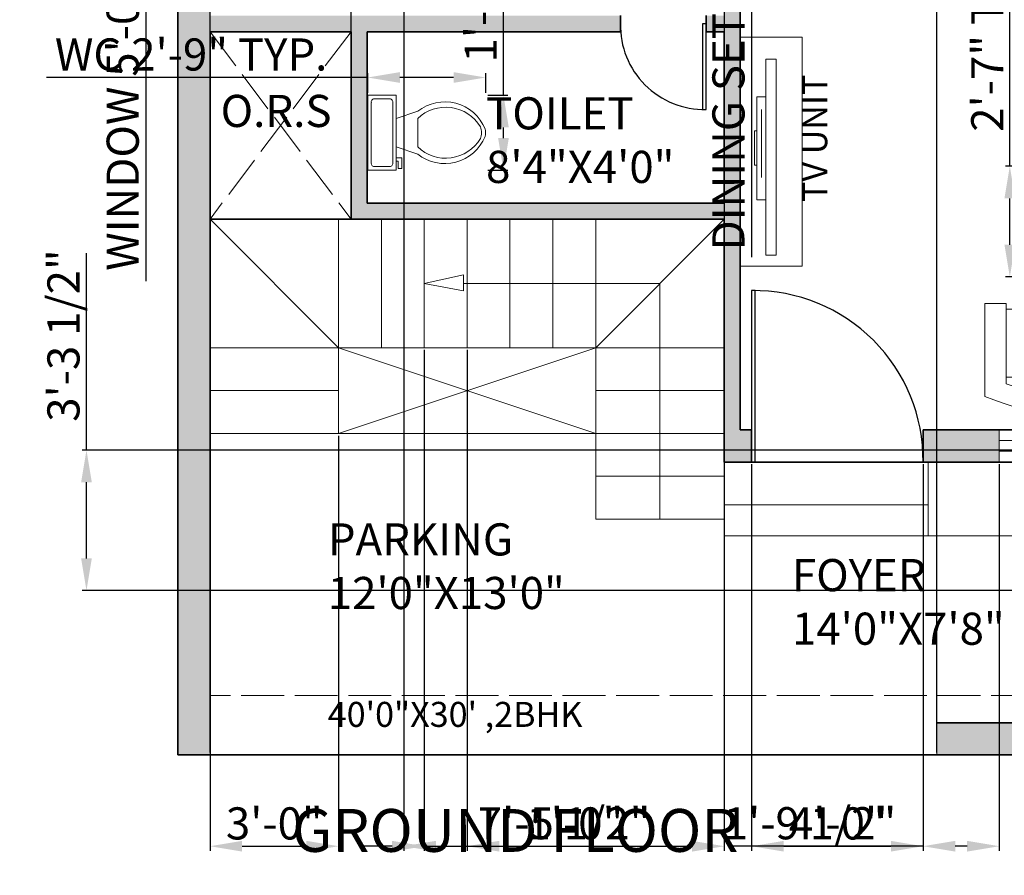
# Model space of a CAD drawing. Units: inches. Extents: x 33024 to 33675, y 11501 to 11939.
# Tile 1 of 3: x 33024 to 33299, y 11501 to 11741. Entities that reach past the tile are written whole.
import ezdxf

# ---------------------------------------------------------------- set-up
doc = ezdxf.new("R2010")
doc.units = ezdxf.units.IN
doc.linetypes.add('ACAD_ISO02W100', pattern=[15, 12, -3])
for name, color, linetype, lineweight in [('A-ANNO-DIMS', 2, 'Continuous', 18), ('A-ANNO-TEXT', 7, 'Continuous', 18), ('A-ANNO-TITL', 7, 'Continuous', 25), ('A-AREA-IDEN', 7, 'Continuous', 18), ('A-DOOR', 4, 'Continuous', 25), ('A-FLOR-FIXT', 9, 'Continuous', 18), ('A-FLOR-OPEN', 8, 'ACAD_ISO02W100', 13), ('A-FLOR-OVHD', 8, 'ACAD_ISO02W100', 13), ('A-FLOR-STRS', 7, 'Continuous', 18), ('A-FURN', 8, 'Continuous', 18), ('A-FURN-FIXD', 8, 'Continuous', 18), ('A-GLAZ', 4, 'Continuous', 18), ('A-WALL', 7, 'Continuous', 35), ('A-WALL-HIDN', 7, 'ACAD_ISO02W100', 18)]:
    doc.layers.add(name, color=color, linetype=linetype, lineweight=lineweight)
doc.layers.add('A-WALL-PATT', color=242, linetype='Continuous', lineweight=13, true_color=0xcd2027)
doc.styles.get("Standard").update_dxf_attribs({"font": 'arial.ttf'})
doc.dimstyles.new('ISO-25', dxfattribs={"dimtxt": 9, "dimasz": 9, "dimexe": 1.25, "dimexo": 0.625, "dimtad": 1, "dimdec": 1, "dimrnd": 9, "dimlunit": 3, "dimtxsty": 'Standard', "dimcen": 2.5, "dimadec": 0, "dimazin": 0, "dimtfac": 1, "dimtdec": 1, "dimtmove": 0, "dimatfit": 3, "dimfxl": 1, "dimarcsym": 0})

# ---------------------------------------------------------------- blocks, each defined once
blk = doc.blocks.new('Toilet - top')
for p, q in [((9.5, -6), (9.5, -2)), ((-8, -8.5), (-8, -8)), ((-7, -8), (-7, -9.5)), ((-4, -8), (-6, -14)), ((4, -8), (6, -14)), ((-10, -8.5), (-8, -8.5)), ((-10, -9.5), (-10, -8.5)), ((-7, -9.5), (-10, -9.5)), ((4, -14), (-4, -14))]:
    blk.add_line(p, q)
blk.add_lwpolyline([(10.5, -8), (10.5, 0), (-10.5, 0), (-10.5, -8)], close=True)
for points in [[(-9.5, -2), (-9.5, -6)], [(8.5, -1), (-8.5, -1)], [(-8.5, -7), (8.5, -7)]]:
    blk.add_lwpolyline(points)
for centre, radius, start, end in [((-8.62, -1.88), 0.884, 81.8699, 188.1301), ((8.62, -1.88), 0.884, 351.8699, 98.1301), ((-8.62, -6.12), 0.884, 171.8699, 278.1301), ((8.62, -6.12), 0.884, 261.8699, 8.1301), ((3.52, -21.58), 12.17, 141.4691, 247.9714), ((4.2, -21.82), 11.33, 136.3677, 238.9468), ((-3.52, -21.58), 12.17, 292.0284, 38.5307), ((-4.2, -21.82), 11.33, 301.053, 43.6321), ((0, -27.88), 4, 245.7318, 294.2682), ((0, -29), 4, 254.8605, 285.1395)]:
    blk.add_arc(centre, radius, start, end)
blk = doc.blocks.new('Sofa - Roundback 7 ft.')
for p, q in [((-12.00002, -32.4421), (-12.00003, -6.5971)), ((11.99997, -32.4421), (11.99998, -6.5971)), ((-36.000027, -34), (-36.000027, -11.4696)), ((-35.999844, -13.3819), (35.9998, -13.3819)), ((35.99998, -34), (35.99998, -11.4696)), ((-36.000027, -32.4421), (35.99998, -32.4421))]:
    blk.add_line(p, q)
for points in [[(-36.000027, -34), (-42.000027, -34), (-42.000027, -8)], [(41.99998, -8), (41.99998, -34), (35.99998, -34)]]:
    blk.add_lwpolyline(points)
for centre, radius, start, end in [((0, -114.25), 114.25, 68.43141, 111.5686), ((-0.00001, -127.1968), 121.1968, 72.72033, 107.2797)]:
    blk.add_arc(centre, radius, start, end)
blk = doc.blocks.new('TV-CONSOLE-64')
for p, q in [((-17.33, 64.14), (-17.33, 0)), ((-7.13, 45.53), (-7.13, 45.53)), ((-7.13, 45.53), (-4.58, 45.53)), ((-4.58, 45.53), (-4.58, 16.72)), ((-5.92, 39.3), (-5.92, 20.26)), ((-4.58, 35.87), (-3.95, 35.87)), ((-3.95, 35.87), (-3.95, 26.18)), ((-3.95, 26.18), (-4.58, 26.18)), ((-4.58, 16.72), (-7.13, 16.72))]:
    blk.add_line(p, q)
blk.add_lwpolyline([(-17.33, 64.14), (0, 64.14), (0, 0), (-17.33, 0)])
blk.add_lwpolyline([(-10.08, 61), (-7.13, 61), (-7.13, 6.14), (-10.08, 6.14)], close=True)
blk = doc.blocks.new('WIN-60X9')
for p, q in [((0, 9), (0, 0)), ((60, 9), (60, 0)), ((60, 6), (0, 6)), ((60, 3), (0, 3))]:
    blk.add_line(p, q)
blk = doc.blocks.new('*D12')
at = {"layer": 'A-ANNO-DIMS', "color": 0, "lineweight": -2, "transparency": 16777216}
for p, q in [((33067.41, 11851.93), (33057.78, 11851.93)), ((33059.03, 11842.93), (33059.03, 11800.93)), ((33067.41, 11791.93), (33057.78, 11791.93)), ((33059.03, 11791.93), (33059.03, 11667.8))]:
    blk.add_line(p, q, dxfattribs=at)
at = {"layer": 'A-ANNO-DIMS', "color": 0, "transparency": 16777216}
for points in [[(33057.53, 11842.93), (33060.53, 11842.93), (33059.03, 11851.93)], [(33057.53, 11800.93), (33060.53, 11800.93), (33059.03, 11791.93)]]:
    blk.add_solid(points, dxfattribs=at)
at = {"layer": 'Defpoints', "color": 0, "transparency": 16777216}
for p in [(33068.03, 11851.93), (33059.03, 11791.93), (33068.03, 11791.93)]:
    blk.add_point(p, dxfattribs=at)
at = {"layer": 'A-ANNO-DIMS', "color": 0, "transparency": 16777216, "insert": (33053.75, 11725.37), "char_height": 9, "attachment_point": 5, "rotation": 90}
blk.add_mtext('WINDOW 5\'-0" TYP.', dxfattribs=at)
blk = doc.blocks.new('*D16')
at = {"layer": 'A-ANNO-DIMS', "color": 0, "lineweight": -2, "transparency": 16777216}
for p, q in [((33121.2, 11724.86), (33031.28, 11724.86)), ((33121.2, 11720.53), (33121.2, 11726.11)), ((33145.25, 11724.86), (33130.2, 11724.86)), ((33154.25, 11720.53), (33154.25, 11726.11))]:
    blk.add_line(p, q, dxfattribs=at)
at = {"layer": 'A-ANNO-DIMS', "color": 0, "transparency": 16777216}
for points in [[(33130.2, 11726.36), (33130.2, 11723.36), (33121.2, 11724.86)], [(33145.25, 11726.36), (33145.25, 11723.36), (33154.25, 11724.86)]]:
    blk.add_solid(points, dxfattribs=at)
at = {"layer": 'Defpoints', "color": 0, "transparency": 16777216}
for p in [(33121.2, 11724.86), (33121.2, 11719.9), (33154.25, 11719.9)]:
    blk.add_point(p, dxfattribs=at)
at = {"layer": 'A-ANNO-DIMS', "color": 0, "transparency": 16777216, "insert": (33071.74, 11730.14), "char_height": 9, "attachment_point": 5}
blk.add_mtext('WC 2\'-9" TYP.', dxfattribs=at)
blk = doc.blocks.new('*D17')
at = {"layer": 'A-ANNO-DIMS', "color": 0, "lineweight": -2, "transparency": 16777216}
for p, q in [((33159.2, 11719.9), (33159.2, 11784.16)), ((33154.87, 11719.9), (33160.45, 11719.9)), ((33159.2, 11707.9), (33159.2, 11710.9)), ((33154.87, 11698.9), (33160.45, 11698.9))]:
    blk.add_line(p, q, dxfattribs=at)
at = {"layer": 'A-ANNO-DIMS', "color": 0, "transparency": 16777216}
for points in [[(33157.7, 11710.9), (33160.7, 11710.9), (33159.2, 11719.9)], [(33157.7, 11707.9), (33160.7, 11707.9), (33159.2, 11698.9)]]:
    blk.add_solid(points, dxfattribs=at)
at = {"layer": 'Defpoints', "color": 0, "transparency": 16777216}
for p in [(33154.25, 11719.9), (33159.2, 11719.9), (33154.25, 11698.9)]:
    blk.add_point(p, dxfattribs=at)
at = {"layer": 'A-ANNO-DIMS', "color": 0, "transparency": 16777216, "insert": (33153.98, 11756.53), "char_height": 9, "attachment_point": 5, "rotation": 90}
blk.add_mtext('1\'-9" TYP.', dxfattribs=at)
blk = doc.blocks.new('*D23')
at = {"layer": 'A-ANNO-DIMS', "color": 0, "lineweight": -2, "transparency": 16777216}
for p, q in [((33301, 11700), (33301, 11765.26)), ((33309.38, 11700), (33299.75, 11700)), ((33301, 11678), (33301, 11691)), ((33309.38, 11669), (33299.75, 11669))]:
    blk.add_line(p, q, dxfattribs=at)
at = {"layer": 'A-ANNO-DIMS', "color": 0, "transparency": 16777216}
for points in [[(33299.5, 11691), (33302.5, 11691), (33301, 11700)], [(33299.5, 11678), (33302.5, 11678), (33301, 11669)]]:
    blk.add_solid(points, dxfattribs=at)
at = {"layer": 'Defpoints', "color": 0, "transparency": 16777216}
for p in [(33301, 11700), (33310, 11700), (33310, 11669)]:
    blk.add_point(p, dxfattribs=at)
at = {"layer": 'A-ANNO-DIMS', "color": 0, "transparency": 16777216, "insert": (33295.85, 11737.13), "char_height": 9, "attachment_point": 5, "rotation": 90}
blk.add_mtext('2\'-7" TYP.', dxfattribs=at)
blk = doc.blocks.new('*D28')
at = {"layer": 'A-ANNO-DIMS', "color": 0, "lineweight": -2, "transparency": 16777216}
for p, q in [((33241.67, 11874.7), (33227.4, 11874.7)), ((33228.65, 11865.7), (33228.65, 11792.7)), ((33241.67, 11783.7), (33227.4, 11783.7)), ((33228.65, 11783.7), (33228.65, 11674.53))]:
    blk.add_line(p, q, dxfattribs=at)
at = {"layer": 'A-ANNO-DIMS', "color": 0, "transparency": 16777216}
for points in [[(33227.15, 11865.7), (33230.15, 11865.7), (33228.65, 11874.7)], [(33227.15, 11792.7), (33230.15, 11792.7), (33228.65, 11783.7)]]:
    blk.add_solid(points, dxfattribs=at)
at = {"layer": 'Defpoints', "color": 0, "transparency": 16777216}
for p in [(33242.3, 11874.7), (33228.65, 11783.7), (33242.3, 11783.7)]:
    blk.add_point(p, dxfattribs=at)
at = {"layer": 'A-ANNO-DIMS', "color": 0, "transparency": 16777216, "insert": (33223.37, 11724.62), "char_height": 9, "attachment_point": 5, "rotation": 90}
blk.add_mtext('DINING SET 7\'-7"', dxfattribs=at)
blk = doc.blocks.new('*D33')
at = {"layer": 'A-ANNO-DIMS', "color": 0, "lineweight": -2, "transparency": 16777216}
for p, q in [((33276.7, 11616.55), (33276.7, 11508.33)), ((33298.03, 11616.55), (33298.03, 11508.33)), ((33276.7, 11509.58), (33222.4, 11509.58)), ((33289.03, 11509.58), (33285.7, 11509.58))]:
    blk.add_line(p, q, dxfattribs=at)
at = {"layer": 'A-ANNO-DIMS', "color": 0, "transparency": 16777216}
for points in [[(33285.7, 11511.08), (33285.7, 11508.08), (33276.7, 11509.58)], [(33289.03, 11511.08), (33289.03, 11508.08), (33298.03, 11509.58)]]:
    blk.add_solid(points, dxfattribs=at)
at = {"layer": 'Defpoints', "color": 0, "transparency": 16777216}
for p in [(33276.7, 11617.18), (33298.03, 11617.18), (33276.7, 11509.58)]:
    blk.add_point(p, dxfattribs=at)
at = {"layer": 'A-ANNO-DIMS', "color": 0, "transparency": 16777216, "insert": (33245.05, 11514.85), "char_height": 9, "attachment_point": 5}
blk.add_mtext('1\'-9 1/2"', dxfattribs=at)
blk = doc.blocks.new('*D34')
at = {"layer": 'A-ANNO-DIMS', "color": 0, "lineweight": -2, "transparency": 16777216}
for p, q in [((33228.7, 11616.55), (33228.7, 11508.33)), ((33276.7, 11616.55), (33276.7, 11508.33)), ((33237.7, 11509.58), (33267.7, 11509.58))]:
    blk.add_line(p, q, dxfattribs=at)
at = {"layer": 'A-ANNO-DIMS', "color": 0, "transparency": 16777216}
for points in [[(33237.7, 11511.08), (33237.7, 11508.08), (33228.7, 11509.58)], [(33267.7, 11511.08), (33267.7, 11508.08), (33276.7, 11509.58)]]:
    blk.add_solid(points, dxfattribs=at)
at = {"layer": 'Defpoints', "color": 0, "transparency": 16777216}
for p in [(33228.7, 11617.18), (33276.7, 11617.18), (33276.7, 11509.58)]:
    blk.add_point(p, dxfattribs=at)
at = {"layer": 'A-ANNO-DIMS', "color": 0, "transparency": 16777216, "insert": (33252.7, 11514.8), "char_height": 9, "attachment_point": 5}
blk.add_mtext('4\'-0"', dxfattribs=at)
blk = doc.blocks.new('*D40')
at = {"layer": 'A-ANNO-DIMS', "color": 0, "lineweight": -2, "transparency": 16777216}
for p, q in [((33077.03, 11535.8), (33077.03, 11922.03)), ((33086.03, 11920.78), (33271.53, 11920.78)), ((33280.53, 11535.8), (33280.53, 11922.03))]:
    blk.add_line(p, q, dxfattribs=at)
at = {"layer": 'A-ANNO-DIMS', "color": 0, "transparency": 16777216}
for points in [[(33086.03, 11922.28), (33086.03, 11919.28), (33077.03, 11920.78)], [(33271.53, 11922.28), (33271.53, 11919.28), (33280.53, 11920.78)]]:
    blk.add_solid(points, dxfattribs=at)
at = {"layer": 'Defpoints', "color": 0, "transparency": 16777216}
for p in [(33280.53, 11920.78), (33077.03, 11535.18), (33280.53, 11535.18)]:
    blk.add_point(p, dxfattribs=at)
at = {"layer": 'A-ANNO-DIMS', "color": 0, "transparency": 16777216, "insert": (33178.78, 11926.05), "char_height": 9, "attachment_point": 5}
blk.add_mtext('16\'-11 1/2"', dxfattribs=at)
blk = doc.blocks.new('*D41')
at = {"layer": 'A-ANNO-DIMS', "color": 0, "lineweight": -2, "transparency": 16777216}
for p, q in [((33077.03, 11624.55), (33077.03, 11508.33)), ((33113.03, 11624.55), (33113.03, 11508.33)), ((33086.03, 11509.58), (33104.03, 11509.58))]:
    blk.add_line(p, q, dxfattribs=at)
at = {"layer": 'A-ANNO-DIMS', "color": 0, "transparency": 16777216}
for points in [[(33086.03, 11511.08), (33086.03, 11508.08), (33077.03, 11509.58)], [(33104.03, 11511.08), (33104.03, 11508.08), (33113.03, 11509.58)]]:
    blk.add_solid(points, dxfattribs=at)
at = {"layer": 'Defpoints', "color": 0, "transparency": 16777216}
for p in [(33077.03, 11625.18), (33113.03, 11625.18), (33113.03, 11509.58)]:
    blk.add_point(p, dxfattribs=at)
at = {"layer": 'A-ANNO-DIMS', "color": 0, "transparency": 16777216, "insert": (33095.03, 11514.8), "char_height": 9, "attachment_point": 5}
blk.add_mtext('3\'-0"', dxfattribs=at)
blk = doc.blocks.new('*D42')
at = {"layer": 'A-ANNO-DIMS', "color": 0, "lineweight": -2, "transparency": 16777216}
for p, q in [((33137.03, 11648.55), (33137.03, 11508.33)), ((33149.03, 11648.55), (33149.03, 11508.33)), ((33128.03, 11509.58), (33119.03, 11509.58)), ((33137.03, 11509.58), (33149.03, 11509.58)), ((33158.03, 11509.58), (33191.36, 11509.58))]:
    blk.add_line(p, q, dxfattribs=at)
at = {"layer": 'A-ANNO-DIMS', "color": 0, "transparency": 16777216}
for points in [[(33128.03, 11511.08), (33128.03, 11508.08), (33137.03, 11509.58)], [(33158.03, 11511.08), (33158.03, 11508.08), (33149.03, 11509.58)]]:
    blk.add_solid(points, dxfattribs=at)
at = {"layer": 'Defpoints', "color": 0, "transparency": 16777216}
for p in [(33137.03, 11649.18), (33149.03, 11649.18), (33149.03, 11509.58)]:
    blk.add_point(p, dxfattribs=at)
at = {"layer": 'A-ANNO-DIMS', "color": 0, "transparency": 16777216, "insert": (33179.2, 11514.8), "char_height": 9, "attachment_point": 5}
blk.add_mtext('1\'-0"', dxfattribs=at)
blk = doc.blocks.new('*D44')
at = {"layer": 'A-ANNO-DIMS', "color": 0, "lineweight": -2, "transparency": 16777216}
for p, q in [((33131.3, 11862.83), (33131.3, 11508.33)), ((33221.03, 11862.83), (33221.03, 11508.33)), ((33140.3, 11509.58), (33212.03, 11509.58))]:
    blk.add_line(p, q, dxfattribs=at)
at = {"layer": 'A-ANNO-DIMS', "color": 0, "transparency": 16777216}
for points in [[(33140.3, 11511.08), (33140.3, 11508.08), (33131.3, 11509.58)], [(33212.03, 11511.08), (33212.03, 11508.08), (33221.03, 11509.58)]]:
    blk.add_solid(points, dxfattribs=at)
at = {"layer": 'Defpoints', "color": 0, "transparency": 16777216}
for p in [(33131.3, 11863.46), (33221.03, 11863.46), (33221.03, 11509.58)]:
    blk.add_point(p, dxfattribs=at)
at = {"layer": 'A-ANNO-DIMS', "color": 0, "transparency": 16777216, "insert": (33176.17, 11514.85), "char_height": 9, "attachment_point": 5}
blk.add_mtext('7\'-5 1/2"', dxfattribs=at)
blk = doc.blocks.new('*D48')
at = {"layer": 'A-ANNO-DIMS', "color": 0, "lineweight": -2, "transparency": 16777216}
for p, q in [((33042.43, 11620.53), (33042.43, 11675.67)), ((33390.91, 11620.53), (33041.18, 11620.53)), ((33042.43, 11590.18), (33042.43, 11611.53)), ((33390.91, 11581.18), (33041.18, 11581.18))]:
    blk.add_line(p, q, dxfattribs=at)
at = {"layer": 'A-ANNO-DIMS', "color": 0, "transparency": 16777216}
for points in [[(33040.93, 11611.53), (33043.93, 11611.53), (33042.43, 11620.53)], [(33040.93, 11590.18), (33043.93, 11590.18), (33042.43, 11581.18)]]:
    blk.add_solid(points, dxfattribs=at)
at = {"layer": 'Defpoints', "color": 0, "transparency": 16777216}
for p in [(33042.43, 11620.53), (33391.53, 11620.53), (33391.53, 11581.18)]:
    blk.add_point(p, dxfattribs=at)
at = {"layer": 'A-ANNO-DIMS', "color": 0, "transparency": 16777216, "insert": (33037.15, 11652.6), "char_height": 9, "attachment_point": 5, "rotation": 90}
blk.add_mtext('3\'-3 1/2"', dxfattribs=at)
blk = doc.blocks.new('*D49')
at = {"layer": 'A-ANNO-DIMS', "color": 0, "lineweight": -2, "transparency": 16777216}
for p, q in [((33077.03, 11685.8), (33077.03, 11922.03)), ((33086.03, 11920.78), (33107.53, 11920.78)), ((33116.53, 11685.8), (33116.53, 11922.03)), ((33116.53, 11920.78), (33171.67, 11920.78))]:
    blk.add_line(p, q, dxfattribs=at)
at = {"layer": 'A-ANNO-DIMS', "color": 0, "transparency": 16777216}
for points in [[(33086.03, 11922.28), (33086.03, 11919.28), (33077.03, 11920.78)], [(33107.53, 11922.28), (33107.53, 11919.28), (33116.53, 11920.78)]]:
    blk.add_solid(points, dxfattribs=at)
at = {"layer": 'Defpoints', "color": 0, "transparency": 16777216}
for p in [(33116.53, 11920.78), (33077.03, 11685.18), (33116.53, 11685.18)]:
    blk.add_point(p, dxfattribs=at)
at = {"layer": 'A-ANNO-DIMS', "color": 0, "transparency": 16777216, "insert": (33148.6, 11926.06), "char_height": 9, "attachment_point": 5}
blk.add_mtext('3\'-3 1/2"', dxfattribs=at)

msp = doc.modelspace()

# ---------------------------------------------------------------- hatches: boundary and pattern name
at = {"layer": 'A-WALL-PATT'}
h = msp.add_hatch(color=256, dxfattribs=at)
h.dxf.hatch_style = 1
h.paths.add_polyline_path([(33548.03, 11895.18), (33068.03, 11895.18), (33068.03, 11851.93), (33077.03, 11851.93), (33077.03, 11886.18), (33221.03, 11886.18), (33221.03, 11794.32, -0.012093), (33223.28, 11794.3), (33225.53, 11794.3), (33225.53, 11886.18), (33382.53, 11886.18), (33382.53, 11845.96, -0.043682), (33382.53, 11826.04), (33382.53, 11810.27), (33384.78, 11810.27, -0.005263), (33385.78, 11810.27), (33387.03, 11810.27), (33387.03, 11886.18), (33539.03, 11886.18), (33539.03, 11851.72), (33548.03, 11851.72)])
h.paths.add_polyline_path([(33077.03, 11791.93), (33068.03, 11791.93), (33068.03, 11535.18), (33077.03, 11535.18), (33077.03, 11544.18), (33077.03, 11737.68), (33116.53, 11737.68), (33116.53, 11685.18), (33221.03, 11685.18), (33221.03, 11617.18), (33228.7, 11617.18), (33228.7, 11626.18), (33225.53, 11626.18), (33225.53, 11746.3), (33221.03, 11746.3), (33221.03, 11742.18), (33215.96, 11742.18), (33215.96, 11737.68), (33221.03, 11737.68), (33221.03, 11689.68), (33121.03, 11689.68), (33121.03, 11737.68), (33179.96, 11737.68), (33191.96, 11737.68), (33191.96, 11738.93, -0.010637), (33191.96, 11739.93), (33191.96, 11742.18), (33179.96, 11742.18), (33077.03, 11742.18)])
h.paths.add_polyline_path([(33548.03, 11791.72), (33539.03, 11791.72), (33539.03, 11758.18), (33426.07, 11758.18), (33414.07, 11758.18), (33414.07, 11755.93, -0.023906), (33414.1, 11753.68), (33426.07, 11753.68), (33487.03, 11753.68), (33487.03, 11705.68), (33387.03, 11705.68), (33387.03, 11753.68), (33390.07, 11753.68), (33390.07, 11754.93), (33390.07, 11755.93), (33390.07, 11758.18), (33387.03, 11758.18), (33387.03, 11762.27), (33382.53, 11762.27), (33382.53, 11701.18), (33387.03, 11701.18), (33491.53, 11701.18), (33491.53, 11753.68), (33539.03, 11753.68), (33539.03, 11581.18), (33498.14, 11581.18), (33498.14, 11572.18), (33539.03, 11572.18), (33539.03, 11544.18), (33280.53, 11544.18), (33280.53, 11535.18), (33548.03, 11535.18)])
h.paths.add_polyline_path([(33391.53, 11626.18), (33391.53, 11626.18), (33391.53, 11665.18), (33382.53, 11665.18), (33382.53, 11626.18), (33358.03, 11626.18), (33358.03, 11617.18), (33382.53, 11617.18), (33382.53, 11572.18), (33387.03, 11572.18), (33438.14, 11572.18), (33438.14, 11581.18), (33391.53, 11581.18), (33391.53, 11614.89)], flags=17)
h = msp.add_hatch(color=256, dxfattribs=at)
h.dxf.hatch_style = 1
h.paths.add_polyline_path([(33298.03, 11626.18), (33276.7, 11626.18), (33276.7, 11618.18, -0.005263), (33276.7, 11617.18), (33298.03, 11617.18)])

# ---------------------------------------------------------------- linework, layer by layer
at = {"layer": 'A-DOOR'}
for p, q in [((33215.96, 11739.93), (33214.96, 11739.93)), ((33214.96, 11739.93), (33214.96, 11715.93)), ((33215.96, 11715.93), (33215.96, 11737.68)), ((33214.96, 11715.93), (33215.96, 11715.93)), ((33229.7, 11665.18), (33228.7, 11665.18)), ((33228.7, 11665.18), (33228.7, 11626.18)), ((33229.7, 11617.18), (33229.7, 11665.18)), ((33228.7, 11617.18), (33229.7, 11617.18))]:
    msp.add_line(p, q, dxfattribs=at)
for centre, radius, start, end in [((33215.46, 11739.43), 23.51, 178.7811, 271.2189), ((33229.2, 11617.68), 47.5, 359.3969, 90.6031)]:
    msp.add_arc(centre, radius, start, end, dxfattribs=at)
at = {"layer": 'A-FLOR-OPEN'}
for p, q in [((33077.03, 11737.68), (33116.53, 11685.18)), ((33116.53, 11737.68), (33077.03, 11685.18))]:
    msp.add_line(p, q, dxfattribs=at)
at = {"layer": 'A-FLOR-OVHD'}
msp.add_line((33382.77, 11551.78), (33077.03, 11551.78), dxfattribs=at)
at = {"layer": 'A-FLOR-STRS'}
for p, q in [((33077.03, 11685.18), (33113.03, 11649.18)), ((33113.03, 11685.18), (33113.03, 11625.18)), ((33125.03, 11685.18), (33125.03, 11649.18)), ((33137.03, 11685.18), (33137.03, 11649.18)), ((33149.03, 11685.18), (33149.03, 11649.18)), ((33161.03, 11685.18), (33161.03, 11649.18)), ((33173.03, 11685.18), (33173.03, 11649.18)), ((33185.03, 11685.18), (33185.03, 11601.18)), ((33221.03, 11685.18), (33185.03, 11649.18)), ((33137.03, 11667.18), (33148.05, 11669.62)), ((33148.05, 11669.62), (33148.05, 11665.16)), ((33148.05, 11665.16), (33137.03, 11667.18)), ((33203.03, 11667.18), (33148.05, 11667.18)), ((33203.03, 11601.18), (33203.03, 11667.18)), ((33221.03, 11649.18), (33077.03, 11649.18)), ((33185.03, 11625.18), (33113.03, 11649.18)), ((33185.03, 11649.18), (33113.03, 11625.18)), ((33113.03, 11637.18), (33077.03, 11637.18)), ((33221.03, 11637.18), (33185.03, 11637.18)), ((33113.03, 11625.18), (33077.03, 11625.18)), ((33113.03, 11625.18), (33185.03, 11625.18)), ((33221.03, 11625.18), (33185.03, 11625.18)), ((33221.03, 11617.18), (33221.03, 11605.18)), ((33221.03, 11613.18), (33185.03, 11613.18)), ((33221.03, 11605.18), (33278.11, 11605.18)), ((33221.03, 11596.48), (33221.03, 11605.18)), ((33221.03, 11601.18), (33185.03, 11601.18)), ((33278.11, 11596.48), (33221.03, 11596.48))]:
    msp.add_line(p, q, dxfattribs=at)
at = {"layer": 'A-FURN-FIXD'}
for p, q in [((33278.11, 11617.18), (33278.11, 11596.48)), ((33278.11, 11596.48), (33382.53, 11596.48))]:
    msp.add_line(p, q, dxfattribs=at)
at = {"layer": 'A-WALL'}
for p, q in [((33068.03, 11895.18), (33068.03, 11535.18)), ((33225.53, 11746.3), (33225.53, 11626.18)), ((33191.96, 11742.18), (33191.96, 11737.68)), ((33215.96, 11742.18), (33215.96, 11737.68)), ((33116.53, 11737.68), (33077.03, 11737.68)), ((33077.03, 11737.68), (33077.03, 11544.18)), ((33116.53, 11737.68), (33116.53, 11685.18)), ((33121.03, 11737.68), (33121.03, 11689.68)), ((33179.96, 11737.68), (33121.03, 11737.68)), ((33191.96, 11737.68), (33179.96, 11737.68)), ((33221.03, 11737.68), (33215.96, 11737.68)), ((33221.03, 11737.68), (33221.03, 11689.68)), ((33221.03, 11689.68), (33121.03, 11689.68)), ((33221.03, 11685.18), (33077.03, 11685.18)), ((33221.03, 11685.18), (33221.03, 11617.18)), ((33228.7, 11626.18), (33225.53, 11626.18)), ((33228.7, 11626.18), (33228.7, 11617.18)), ((33382.53, 11626.18), (33276.7, 11626.18)), ((33276.7, 11626.18), (33276.7, 11617.18)), ((33382.53, 11617.18), (33221.03, 11617.18)), ((33280.53, 11544.18), (33539.03, 11544.18)), ((33068.03, 11535.18), (33548.03, 11535.18))]:
    msp.add_line(p, q, dxfattribs=at)
at = {"layer": 'A-WALL-HIDN'}
for p, q in [((33077.03, 11544.18), (33077.03, 11535.18)), ((33280.53, 11544.18), (33280.53, 11535.18))]:
    msp.add_line(p, q, dxfattribs=at)

# ---------------------------------------------------------------- block references
at = {"layer": 'A-FLOR-FIXT', "rotation": 89.99999999999999}
msp.add_blockref('Toilet - top', (33121.2, 11709.4), dxfattribs=at)
at = {"layer": 'A-FURN', "rotation": 180}
msp.add_blockref('Sofa - Roundback 7 ft.', (33336, 11627.56), dxfattribs=at)
at = {"layer": 'A-FURN-FIXD', "rotation": 180}
msp.add_blockref('TV-CONSOLE-64', (33225.53, 11736.14), dxfattribs=at)
at = {"layer": 'A-GLAZ'}
msp.add_blockref('WIN-60X9', (33298.03, 11617.18), dxfattribs=at)

# ---------------------------------------------------------------- texts
at = {"layer": 'A-ANNO-TEXT', "insert": (33242.86, 11690), "char_height": 7, "attachment_point": 1, "rotation": 90}
msp.add_mtext_dynamic_manual_height_columns('TV UNIT', width=70, gutter_width=12.5, heights=[0], dxfattribs=at)
at = {"layer": 'A-ANNO-TITL', "attachment_point": 1}
for s, width, insert, char_height in [('40\'0"X30\' ,2BHK', 93.1388, (33110, 11550), 7), ('GROUND FLOOR', 290, (33100, 11520), 12)]:
    msp.add_mtext_dynamic_manual_height_columns(s, width=width, gutter_width=12.5, heights=[0], dxfattribs=dict(at, insert=insert, char_height=char_height))
at = {"layer": 'A-AREA-IDEN', "char_height": 9, "attachment_point": 1}
for s, insert in [('O.R.S', (33080, 11720)), ('TOILET\\P8\'4"X4\'0"', (33154.33, 11719.33)), ('PARKING\\P12\'0"X13\'0"', (33110, 11600)), ('FOYER\\P14\'0"X7\'8"', (33240, 11590))]:
    msp.add_mtext_dynamic_manual_height_columns(s, width=70, gutter_width=12.5, heights=[0], dxfattribs=dict(at, insert=insert))

# ---------------------------------------------------------------- dimensions: what is measured, and where the dimension line sits
at = {"layer": 'A-ANNO-DIMS'}
for base, p1, p2, picture, middle in [((33280.53, 11920.78), (33077.03, 11535.18), (33280.53, 11535.18), '*D40', (33178.78, 11926.05)), ((33116.53, 11920.78), (33077.03, 11685.18), (33116.53, 11685.18), '*D49', (33148.6, 11926.06)), ((33221.03, 11509.58), (33131.3, 11863.46), (33221.03, 11863.46), '*D44', (33176.17, 11514.85)), ((33149.03, 11509.58), (33137.03, 11649.18), (33149.03, 11649.18), '*D42', (33179.2, 11514.8)), ((33113.03, 11509.58), (33077.03, 11625.18), (33113.03, 11625.18), '*D41', (33095.03, 11514.8)), ((33276.7, 11509.58), (33298.03, 11617.18), (33276.7, 11617.18), '*D33', (33245.05, 11514.85)), ((33276.7, 11509.58), (33228.7, 11617.18), (33276.7, 11617.18), '*D34', (33252.7, 11514.8))]:
    dim = msp.add_linear_dim(base=base, p1=p1, p2=p2, dimstyle='ISO-25', override={"dimdec": 1, "dimlfac": 1, "dimrnd": 0, "dimzin": 1, "dimdsep": 46, "dimlunit": 4, "dimfrac": 2}, dxfattribs=at)
    dim.commit()
    dim.dimension.update_dxf_attribs({"geometry": picture, "text_midpoint": middle})
for base, p1, p2, angle, text, picture, middle in [((33228.65, 11783.7), (33242.3, 11874.7), (33242.3, 11783.7), 270, 'DINING SET <>', '*D28', (33223.37, 11724.62)), ((33059.03, 11791.93), (33068.03, 11851.93), (33068.03, 11791.93), 270, 'WINDOW <> TYP.', '*D12', (33053.75, 11725.37)), ((33159.2, 11719.9), (33154.25, 11698.9), (33154.25, 11719.9), 90, '<> TYP.', '*D17', (33153.98, 11756.53)), ((33301, 11700), (33310, 11669), (33310, 11700), 90, '<> TYP.', '*D23', (33295.85, 11737.13)), ((33121.2009, 11724.8592), (33154.2472, 11719.9023), (33121.2009, 11719.9023), 180, 'WC <> TYP.', '*D16', (33071.742, 11730.1377))]:
    dim = msp.add_linear_dim(base=base, p1=p1, p2=p2, angle=angle, text=text, dimstyle='ISO-25', override={"dimdec": 1, "dimlfac": 1, "dimrnd": 0, "dimzin": 1, "dimdsep": 46, "dimlunit": 4, "dimfrac": 2}, dxfattribs=at)
    dim.commit()
    dim.dimension.update_dxf_attribs({"geometry": picture, "text_midpoint": middle})
dim = msp.add_linear_dim(base=(33042.4322, 11620.5337), p1=(33391.5322, 11581.1761), p2=(33391.5322, 11620.5337), angle=90, dimstyle='ISO-25', override={"dimdec": 1, "dimlfac": 1, "dimrnd": 0, "dimzin": 1, "dimdsep": 46, "dimlunit": 4, "dimfrac": 2}, dxfattribs=at)
dim.commit()
dim.dimension.update_dxf_attribs({"geometry": '*D48', "text_midpoint": (33037.1507, 11652.6034)})

doc.saveas('drawing.dxf')
